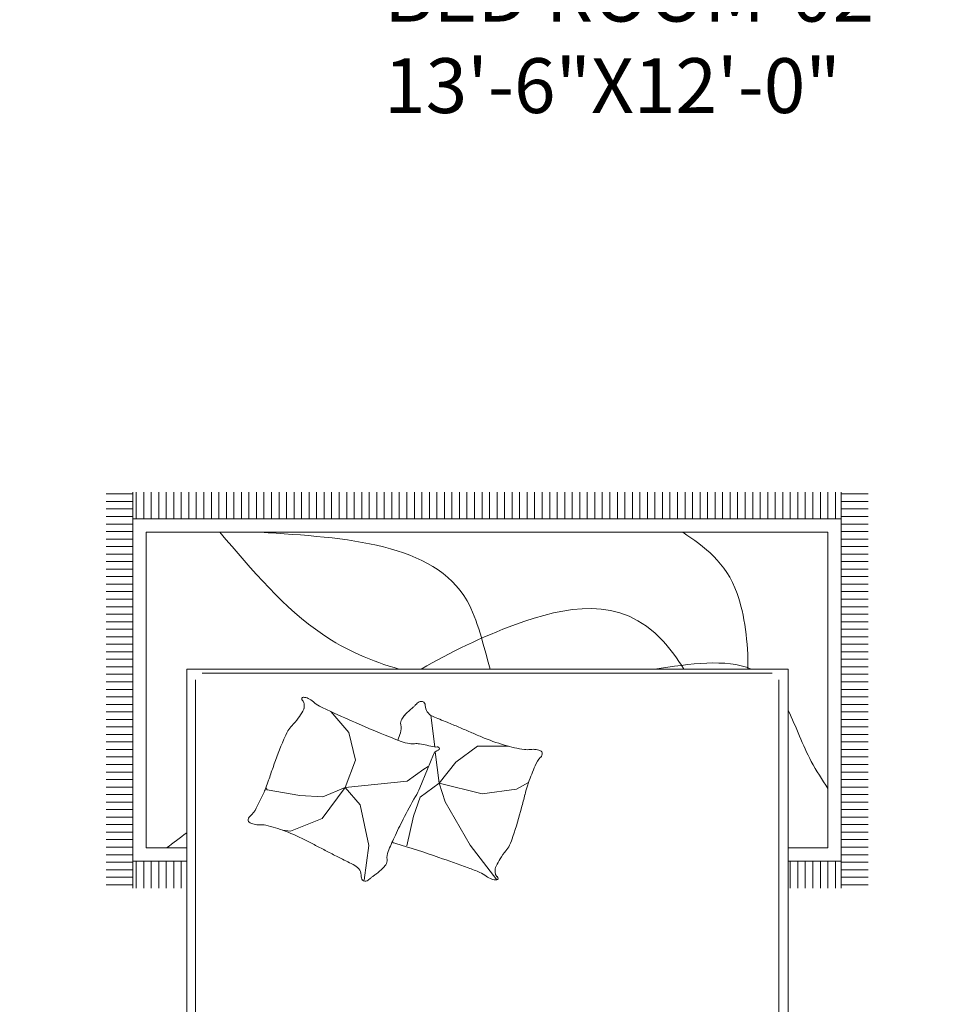
# Model space of a CAD drawing. Units: inches. Extents: x -7 to 1228, y -146 to 1091.
# Tile 18 of 88: x 425 to 511, y 103 to 194. Entities that reach past the tile are written whole.
import ezdxf

# ---------------------------------------------------------------- set-up
doc = ezdxf.new("R2010")
doc.units = ezdxf.units.IN
doc.layers.add('A-AREA-IDEN', color=7, linetype='Continuous', lineweight=18)
doc.layers.add('A-FURN', color=8, linetype='Continuous', lineweight=18)
doc.styles.add('DIM_FONT', font='SIMPLEX.shx', dxfattribs={"width": 0.8})
doc.styles.get("Standard").update_dxf_attribs({"font": 'arial.ttf'})

# ---------------------------------------------------------------- blocks, each defined once
blk = doc.blocks.new('A$C4F634EDD')
for p, q in [((0, 2.6295), (0, 2.2295)), ((0.5, 2.6295), (0, 2.6295)), ((0.5, 2.6295), (2.3, 2.6295)), ((0.5, 0.5295), (0.5, 2.6295)), ((0.5, 2.2295), (0.5, 2.6295)), ((2.3, 2.6295), (2.3, 0.5295)), ((2.3, 2.6295), (2.8, 2.6295)), ((2.3, 2.2295), (2.3, 2.6295)), ((2.8, 2.6295), (2.8, 2.2295)), ((0.2457, 2.5697), (0.2457, 2.4733)), ((0.5, 2.5771), (2.3, 2.5771)), ((2.392, 2.5115), (2.5692, 2.5765)), ((2.5692, 2.5765), (2.574, 2.5743)), ((2.574, 2.5743), (2.6638, 2.3298)), ((2.4946, 2.5331), (2.4985, 2.5445)), ((2.4985, 2.5445), (2.5516, 2.564)), ((2.5062, 2.5454), (2.5004, 2.5392)), ((2.5004, 2.5392), (2.5013, 2.5315)), ((2.5062, 2.5454), (2.5487, 2.561)), ((2.5235, 2.5256), (2.5062, 2.5454)), ((2.5483, 2.5347), (2.5487, 2.561)), ((2.5487, 2.561), (2.5571, 2.56)), ((2.5615, 2.5536), (2.5514, 2.5318)), ((2.5516, 2.564), (2.5637, 2.5584)), ((2.5571, 2.56), (2.5615, 2.5536)), ((2.5615, 2.5536), (2.5791, 2.5058)), ((2.5637, 2.5584), (2.6418, 2.3458)), ((2.3898, 2.5066), (2.392, 2.5115)), ((2.4795, 2.2621), (2.3898, 2.5066)), ((2.412, 2.5007), (2.4634, 2.5196)), ((2.4634, 2.5196), (2.4875, 2.454)), ((2.4842, 2.5232), (2.47, 2.518)), ((2.47, 2.518), (2.472, 2.5127)), ((2.472, 2.5127), (2.4862, 2.5179)), ((2.4881, 2.5126), (2.4739, 2.5074)), ((2.4739, 2.5074), (2.4759, 2.502)), ((2.4759, 2.502), (2.4901, 2.5073)), ((2.4862, 2.5179), (2.4842, 2.5232)), ((2.4901, 2.5073), (2.4881, 2.5126)), ((2.5734, 2.3187), (2.4946, 2.5331)), ((2.5013, 2.5315), (2.5188, 2.4836)), ((2.5013, 2.5315), (2.5231, 2.5214)), ((2.5231, 2.5214), (2.5235, 2.5256)), ((2.5523, 2.4417), (2.5231, 2.5214)), ((2.5483, 2.5347), (2.5235, 2.5256)), ((2.5514, 2.5318), (2.5483, 2.5347)), ((2.5807, 2.4521), (2.5514, 2.5318)), ((2.5791, 2.5058), (2.5788, 2.4956)), ((2.4361, 2.4352), (2.412, 2.5007)), ((2.492, 2.5019), (2.4778, 2.4967)), ((2.4778, 2.4967), (2.4798, 2.4914)), ((2.4798, 2.4914), (2.494, 2.4966)), ((2.4959, 2.4913), (2.4817, 2.4861)), ((2.4817, 2.4861), (2.4837, 2.4808)), ((2.4837, 2.4808), (2.4979, 2.486)), ((2.4998, 2.4807), (2.4856, 2.4755)), ((2.494, 2.4966), (2.492, 2.5019)), ((2.4979, 2.486), (2.4959, 2.4913)), ((2.5018, 2.4754), (2.4998, 2.4807)), ((2.5188, 2.4836), (2.5256, 2.4761)), ((2.5788, 2.4956), (2.5767, 2.4848)), ((2.5767, 2.4848), (2.5795, 2.4717)), ((2.4875, 2.454), (2.4361, 2.4352)), ((2.4856, 2.4755), (2.4876, 2.4702)), ((2.4876, 2.4702), (2.5018, 2.4754)), ((2.5037, 2.47), (2.4895, 2.4648)), ((2.4895, 2.4648), (2.4915, 2.4595)), ((2.4915, 2.4595), (2.5057, 2.4647)), ((2.5057, 2.4647), (2.5037, 2.47)), ((2.5256, 2.4761), (2.5342, 2.4692)), ((2.5342, 2.4692), (2.5405, 2.4574)), ((2.5405, 2.4574), (2.547, 2.4397)), ((2.5795, 2.4717), (2.586, 2.454)), ((2.5807, 2.4521), (2.6158, 2.3564)), ((2.5984, 2.4204), (2.586, 2.454)), ((0.0957, 2.4197), (0.192, 2.4197)), ((0.2994, 2.4197), (0.3957, 2.4197)), ((2.4457, 2.4146), (2.4563, 2.4185)), ((2.4563, 2.4185), (2.4602, 2.4078)), ((2.4634, 2.4211), (2.474, 2.425)), ((2.4673, 2.4104), (2.4634, 2.4211)), ((2.474, 2.425), (2.4779, 2.4143)), ((2.4811, 2.4276), (2.4917, 2.4315)), ((2.485, 2.4169), (2.4811, 2.4276)), ((2.4956, 2.4208), (2.485, 2.4169)), ((2.4917, 2.4315), (2.4956, 2.4208)), ((2.5594, 2.4061), (2.547, 2.4397)), ((2.5523, 2.4417), (2.5875, 2.346)), ((2.6047, 2.4086), (2.5984, 2.4204)), ((2.4496, 2.4039), (2.4457, 2.4146)), ((2.4602, 2.4078), (2.4496, 2.4039)), ((2.4528, 2.3951), (2.4635, 2.399)), ((2.4567, 2.3844), (2.4528, 2.3951)), ((2.4674, 2.3883), (2.4567, 2.3844)), ((2.4635, 2.399), (2.4674, 2.3883)), ((2.4779, 2.4143), (2.4673, 2.4104)), ((2.4706, 2.4016), (2.4812, 2.4055)), ((2.4745, 2.3909), (2.4706, 2.4016)), ((2.4851, 2.3949), (2.4745, 2.3909)), ((2.4812, 2.4055), (2.4851, 2.3949)), ((2.4883, 2.4081), (2.4989, 2.412)), ((2.4922, 2.3975), (2.4883, 2.4081)), ((2.5028, 2.4014), (2.4922, 2.3975)), ((2.4954, 2.3886), (2.5061, 2.3925)), ((2.4993, 2.378), (2.4954, 2.3886)), ((2.4989, 2.412), (2.5028, 2.4014)), ((2.5061, 2.3925), (2.51, 2.3819)), ((2.5622, 2.393), (2.5594, 2.4061)), ((2.5601, 2.3822), (2.5622, 2.393)), ((2.6133, 2.4017), (2.6047, 2.4086)), ((2.6201, 2.3941), (2.6133, 2.4017)), ((2.6376, 2.3463), (2.6201, 2.3941)), ((2.6499, 2.3979), (2.6397, 2.3953)), ((2.6417, 2.39), (2.6488, 2.391)), ((2.6488, 2.391), (2.6538, 2.3895)), ((2.6551, 2.397), (2.6499, 2.3979)), ((2.6538, 2.3895), (2.6596, 2.388)), ((2.6627, 2.392), (2.6551, 2.397)), ((2.6596, 2.388), (2.6626, 2.3867)), ((2.6626, 2.3867), (2.6662, 2.388)), ((2.6692, 2.394), (2.6627, 2.392)), ((2.6662, 2.388), (2.6632, 2.3828)), ((2.6736, 2.3944), (2.6692, 2.394)), ((2.6765, 2.391), (2.6736, 2.3944)), ((2.6742, 2.3795), (2.6765, 2.391)), ((0.2457, 2.366), (0.2457, 2.2697)), ((2.46, 2.3756), (2.4706, 2.3795)), ((2.4639, 2.365), (2.46, 2.3756)), ((2.4745, 2.3689), (2.4639, 2.365)), ((2.4672, 2.3561), (2.4778, 2.36)), ((2.4706, 2.3795), (2.4745, 2.3689)), ((2.4777, 2.3821), (2.4883, 2.386)), ((2.4816, 2.3715), (2.4777, 2.3821)), ((2.4778, 2.36), (2.4817, 2.3494)), ((2.4922, 2.3754), (2.4816, 2.3715)), ((2.4849, 2.3626), (2.4955, 2.3665)), ((2.4888, 2.352), (2.4849, 2.3626)), ((2.4883, 2.386), (2.4922, 2.3754)), ((2.4955, 2.3665), (2.4994, 2.3559)), ((2.51, 2.3819), (2.4993, 2.378)), ((2.5026, 2.3691), (2.5132, 2.373)), ((2.5065, 2.3585), (2.5026, 2.3691)), ((2.5171, 2.3624), (2.5065, 2.3585)), ((2.5132, 2.373), (2.5171, 2.3624)), ((2.5238, 2.3769), (2.538, 2.3821)), ((2.5277, 2.3663), (2.5238, 2.3769)), ((2.5419, 2.3715), (2.5277, 2.3663)), ((2.538, 2.3821), (2.5419, 2.3715)), ((2.5598, 2.372), (2.5601, 2.3822)), ((2.5774, 2.3242), (2.5598, 2.372)), ((2.6632, 2.3828), (2.6736, 2.3744)), ((2.6736, 2.3744), (2.6922, 2.3593)), ((2.6824, 2.3858), (2.6742, 2.3795)), ((2.6873, 2.3815), (2.6824, 2.3858)), ((2.6853, 2.369), (2.6873, 2.3815)), ((2.6946, 2.376), (2.6853, 2.369)), ((2.6922, 2.3593), (2.7051, 2.3473)), ((2.6995, 2.3713), (2.6946, 2.376)), ((2.695, 2.3603), (2.6995, 2.3713)), ((2.7031, 2.3682), (2.695, 2.3603)), ((2.7096, 2.3616), (2.7031, 2.3682)), ((2.7062, 2.351), (2.7096, 2.3616)), ((0, 2.3301), (0.5, 2.3301)), ((2.8, 2.3301), (2.3, 2.3301)), ((2.4711, 2.3455), (2.4672, 2.3561)), ((2.4817, 2.3494), (2.4711, 2.3455)), ((2.4994, 2.3559), (2.4888, 2.352)), ((2.5774, 2.3242), (2.5875, 2.346)), ((2.5875, 2.346), (2.5905, 2.3431)), ((2.5905, 2.3431), (2.5901, 2.3168)), ((2.6154, 2.3522), (2.5905, 2.3431)), ((2.613, 2.3312), (2.6077, 2.3293)), ((2.6077, 2.3293), (2.6135, 2.3141)), ((2.6192, 2.3174), (2.613, 2.3312)), ((2.6153, 2.3261), (2.6327, 2.3324)), ((2.6158, 2.3564), (2.6154, 2.3522)), ((2.6154, 2.3522), (2.6327, 2.3324)), ((2.6376, 2.3463), (2.6158, 2.3564)), ((2.6369, 2.332), (2.6161, 2.3243)), ((2.6327, 2.3324), (2.6385, 2.3386)), ((2.6418, 2.3458), (2.6369, 2.332)), ((2.6385, 2.3386), (2.6376, 2.3463)), ((2.6638, 2.3298), (2.6616, 2.3249)), ((2.7051, 2.3473), (2.7079, 2.3475)), ((2.7147, 2.3578), (2.7062, 2.351)), ((2.7079, 2.3475), (2.7079, 2.3443)), ((2.7079, 2.3443), (2.727, 2.3277)), ((2.7214, 2.3517), (2.7147, 2.3578)), ((2.7196, 2.34), (2.7214, 2.3517)), ((2.7286, 2.3466), (2.7196, 2.34)), ((2.7346, 2.3423), (2.7286, 2.3466)), ((2.732, 2.3295), (2.7346, 2.3423)), ((2.7423, 2.3345), (2.732, 2.3295)), ((2.7495, 2.325), (2.7423, 2.3345)), ((2.6172, 2.3086), (2.4844, 2.2599)), ((2.5362, 2.305), (2.5185, 2.2985)), ((2.5401, 2.2944), (2.5362, 2.305)), ((2.561, 2.3141), (2.5433, 2.3076)), ((2.5433, 2.3076), (2.5472, 2.297)), ((2.5472, 2.297), (2.5649, 2.3035)), ((2.5649, 2.3035), (2.561, 2.3141)), ((2.5855, 2.3131), (2.5734, 2.3187)), ((2.5818, 2.3178), (2.5774, 2.3242)), ((2.5901, 2.3168), (2.5818, 2.3178)), ((2.6104, 2.3222), (2.5855, 2.3131)), ((2.5901, 2.3168), (2.6097, 2.324)), ((2.6135, 2.3141), (2.6244, 2.2977)), ((2.626, 2.3069), (2.6192, 2.3174)), ((2.6616, 2.3249), (2.6234, 2.3109)), ((2.6365, 2.2916), (2.626, 2.3069)), ((2.727, 2.3277), (2.7512, 2.2983)), ((2.7406, 2.3172), (2.7495, 2.325)), ((2.7519, 2.3218), (2.7406, 2.3172)), ((2.7575, 2.3144), (2.7519, 2.3218)), ((2.7526, 2.3045), (2.7575, 2.3144)), ((2.7622, 2.308), (2.7526, 2.3045)), ((2.7574, 2.2924), (2.7673, 2.2997)), ((2.7673, 2.2997), (2.7622, 2.308)), ((0.5953, 2.1912), (0.616, 2.2738)), ((1.4546, 2.1912), (1.4752, 2.2738)), ((2.5114, 2.2959), (2.4936, 2.2894)), ((2.4936, 2.2894), (2.4976, 2.2788)), ((2.4976, 2.2788), (2.5153, 2.2853)), ((2.5153, 2.2853), (2.5114, 2.2959)), ((2.5185, 2.2985), (2.5224, 2.2879)), ((2.5224, 2.2879), (2.5401, 2.2944)), ((2.6244, 2.2977), (2.6349, 2.2825)), ((2.6349, 2.2825), (2.638, 2.273)), ((2.6407, 2.2834), (2.6365, 2.2916)), ((2.6399, 2.2712), (2.6374, 2.2659)), ((2.638, 2.273), (2.6399, 2.2712)), ((2.6438, 2.2739), (2.6407, 2.2834)), ((2.6519, 2.2716), (2.6438, 2.2739)), ((2.6535, 2.2628), (2.6519, 2.2716)), ((2.7512, 2.2983), (2.756, 2.2695)), ((2.7687, 2.2905), (2.7574, 2.2924)), ((2.7587, 2.279), (2.7699, 2.2828)), ((2.7708, 2.2725), (2.7587, 2.279)), ((2.7699, 2.2828), (2.7687, 2.2905)), ((2.7706, 2.2643), (2.7708, 2.2725)), ((2.4844, 2.2599), (2.4795, 2.2621)), ((2.6374, 2.2659), (2.6398, 2.257)), ((2.6398, 2.257), (2.6509, 2.259)), ((2.6509, 2.259), (2.6431, 2.2492)), ((2.6431, 2.2492), (2.6473, 2.2398)), ((2.6473, 2.2398), (2.6592, 2.2429)), ((2.6592, 2.2429), (2.6521, 2.2314)), ((2.6636, 2.2409), (2.6535, 2.2628)), ((2.6836, 2.2287), (2.6636, 2.2409)), ((2.7459, 2.2483), (2.7284, 2.2317)), ((2.756, 2.2695), (2.7459, 2.2483)), ((2.7509, 2.2314), (2.7459, 2.2418)), ((2.7459, 2.2418), (2.7568, 2.2352)), ((2.7529, 2.2505), (2.7645, 2.2498)), ((2.7607, 2.2424), (2.7529, 2.2505)), ((2.7568, 2.2352), (2.7607, 2.2424)), ((2.759, 2.2637), (2.7706, 2.2643)), ((2.7676, 2.2559), (2.759, 2.2637)), ((2.7645, 2.2498), (2.7676, 2.2559)), ((0, 2.2295), (0.5, 2.2295)), ((2.8, 2.2295), (2.3, 2.2295)), ((2.6521, 2.2314), (2.6598, 2.2248)), ((2.6598, 2.2248), (2.6697, 2.2309)), ((2.6697, 2.2309), (2.6684, 2.219)), ((2.6684, 2.219), (2.6761, 2.2145)), ((2.6761, 2.2145), (2.6821, 2.2237)), ((2.6821, 2.2237), (2.6843, 2.2135)), ((2.7063, 2.2256), (2.6836, 2.2287)), ((2.6843, 2.2135), (2.6927, 2.2117)), ((2.6927, 2.2117), (2.6986, 2.222)), ((2.6986, 2.222), (2.7019, 2.2098)), ((2.7284, 2.2317), (2.7063, 2.2256)), ((2.7102, 2.2104), (2.7113, 2.2218)), ((2.7113, 2.2218), (2.7192, 2.2137)), ((2.7192, 2.2137), (2.7255, 2.2152)), ((2.7255, 2.2152), (2.7242, 2.2265)), ((2.7242, 2.2265), (2.7324, 2.2165)), ((2.7324, 2.2165), (2.7386, 2.2208)), ((2.7386, 2.2208), (2.7354, 2.2306)), ((2.7354, 2.2306), (2.7462, 2.2264)), ((2.7462, 2.2264), (2.7509, 2.2314)), ((0.5878, 2.1612), (0.5953, 2.1912)), ((1.4471, 2.1612), (1.4546, 2.1912)), ((2.7019, 2.2098), (2.7102, 2.2104)), ((1.5035, 2.141), (0.5458, 2.141)), ((1.5035, 2.141), (2.2716, 1.7136)), ((0.5258, 2.121), (0.5258, 0.5617)), ((1.576, 1.9433), (1.5624, 1.8479)), ((0.5458, 1.8684), (1.5653, 1.8684)), ((1.5624, 1.8479), (1.5641, 1.7178)), ((2.2716, 0.5617), (2.2716, 1.7136)), ((0.3386, 0), (0.3386, 1.1852)), ((0.3486, 1.1052), (0.3486, 1.1852)), ((0.3711, 1.1052), (0.3711, 1.1852)), ((0.3936, 1.1052), (0.3936, 1.1852)), ((0.4161, 1.1052), (0.4161, 1.1852)), ((0.4386, 1.1052), (0.4386, 1.1852)), ((0.4611, 1.1052), (0.4611, 1.1852)), ((0.4836, 1.1052), (0.4836, 1.1852)), ((2.3061, 1.1052), (2.3061, 1.1852)), ((2.3286, 1.1052), (2.3286, 1.1852)), ((2.3511, 1.1052), (2.3511, 1.1852)), ((2.3736, 1.1052), (2.3736, 1.1852)), ((2.3961, 1.1052), (2.3961, 1.1852)), ((2.4186, 1.1052), (2.4186, 1.1852)), ((2.4411, 1.1052), (2.4411, 1.1852)), ((2.4588, 1.1852), (2.4588, 0)), ((0.2586, 1.1753), (0.3386, 1.1753)), ((0.2586, 1.1528), (0.3386, 1.1528)), ((1.031, 1.1612), (1.0448, 1.0581)), ((1.4276, 1.1611), (1.3484, 1.0571)), ((2.4588, 1.1753), (2.5388, 1.1753)), ((2.4588, 1.1528), (2.5388, 1.1528)), ((0.2586, 1.1303), (0.3386, 1.1303)), ((2.4588, 1.1303), (2.5388, 1.1303)), ((0.2586, 1.1078), (0.3386, 1.1078)), ((0.3386, 1.1052), (0.5, 1.1052)), ((2.3, 1.1052), (2.4588, 1.1052)), ((2.4588, 1.1078), (2.5388, 1.1078)), ((0.2586, 1.0853), (0.3386, 1.0853)), ((0.2586, 1.0628), (0.3386, 1.0628)), ((0.3786, 1.0652), (0.5, 1.0652)), ((0.3786, 0.12), (0.3786, 1.0652)), ((2.3, 1.0652), (2.4188, 1.0652)), ((2.4188, 1.0652), (2.4188, 0.12)), ((2.4588, 1.0853), (2.5388, 1.0853)), ((2.4588, 1.0628), (2.5388, 1.0628)), ((0.2586, 1.0403), (0.3386, 1.0403)), ((1.0448, 1.0581), (1.019, 0.936)), ((1.1784, 0.9702), (1.1586, 1.0591)), ((1.3484, 1.0571), (1.2733, 0.9268)), ((2.4588, 1.0403), (2.5388, 1.0403)), ((0.2586, 1.0178), (0.3386, 1.0178)), ((0.8108, 1.0151), (0.7868, 1.0117)), ((0.9054, 0.9773), (0.8108, 1.0151)), ((2.4588, 1.0178), (2.5388, 1.0178)), ((0.2586, 0.9953), (0.3386, 0.9953)), ((0.9743, 0.8845), (0.9054, 0.9773)), ((2.4588, 0.9953), (2.5388, 0.9953)), ((0.2586, 0.9728), (0.3386, 0.9728)), ((0.2586, 0.9503), (0.3386, 0.9503)), ((1.1982, 0.9129), (1.1784, 0.9702)), ((2.4588, 0.9728), (2.5388, 0.9728)), ((2.4588, 0.9503), (2.5388, 0.9503)), ((0.2586, 0.9278), (0.3386, 0.9278)), ((1.019, 0.936), (0.9743, 0.8845)), ((1.2733, 0.9268), (1.2555, 0.8715)), ((2.4588, 0.9278), (2.5388, 0.9278)), ((0.2586, 0.9053), (0.3386, 0.9053)), ((0.7403, 0.8913), (0.737, 0.8849)), ((0.8384, 0.9085), (0.7403, 0.8913)), ((0.9072, 0.912), (0.8384, 0.9085)), ((0.9743, 0.8845), (0.9072, 0.912)), ((0.9743, 0.8845), (1.0052, 0.802)), ((0.9743, 0.8845), (1.16, 0.8656)), ((1.1973, 0.8853), (1.2203, 0.829)), ((1.2555, 0.8715), (1.1982, 0.9129)), ((1.2555, 0.8715), (1.384, 0.9031)), ((1.384, 0.9031), (1.4868, 0.8892)), ((1.4868, 0.8892), (1.5228, 0.8692)), ((2.4588, 0.9053), (2.5388, 0.9053)), ((0.2586, 0.8828), (0.3386, 0.8828)), ((0.2586, 0.8603), (0.3386, 0.8603)), ((1.16, 0.8656), (1.2099, 0.8295)), ((1.2555, 0.8715), (1.2437, 0.7773)), ((1.2555, 0.8715), (1.3049, 0.8082)), ((2.4588, 0.8828), (2.5388, 0.8828)), ((2.4588, 0.8603), (2.5388, 0.8603)), ((0.2586, 0.8378), (0.3386, 0.8378)), ((1.2099, 0.8295), (1.222, 0.8209)), ((1.2203, 0.829), (1.2381, 0.7855)), ((2.4588, 0.8378), (2.5388, 0.8378)), ((0.2586, 0.8153), (0.3386, 0.8153)), ((1.0052, 0.802), (0.9846, 0.7194)), ((1.3049, 0.8082), (1.3701, 0.7608)), ((2.4588, 0.8153), (2.5388, 0.8153)), ((0.2586, 0.7928), (0.3386, 0.7928)), ((0.2586, 0.7703), (0.3386, 0.7703)), ((2.4588, 0.7928), (2.5388, 0.7928)), ((2.4588, 0.7703), (2.5388, 0.7703)), ((0.2586, 0.7478), (0.3386, 0.7478)), ((1.2419, 0.7626), (1.23, 0.668)), ((1.3701, 0.7608), (1.463, 0.7608)), ((2.4588, 0.7478), (2.5388, 0.7478)), ((0.2586, 0.7253), (0.3386, 0.7253)), ((0.9846, 0.7194), (0.931, 0.6569)), ((2.4588, 0.7253), (2.5388, 0.7253)), ((0.2586, 0.7028), (0.3386, 0.7028)), ((0.2586, 0.6803), (0.3386, 0.6803)), ((2.4588, 0.7028), (2.5388, 0.7028)), ((2.4588, 0.6803), (2.5388, 0.6803)), ((0.2586, 0.6578), (0.3386, 0.6578)), ((2.4588, 0.6578), (2.5388, 0.6578)), ((0.2586, 0.6353), (0.3386, 0.6353)), ((2.4588, 0.6353), (2.5388, 0.6353)), ((0.2586, 0.6128), (0.3386, 0.6128)), ((0.2586, 0.5903), (0.3386, 0.5903)), ((2.4588, 0.6128), (2.5388, 0.6128)), ((2.4588, 0.5903), (2.5388, 0.5903)), ((0.2586, 0.5678), (0.3386, 0.5678)), ((2.4588, 0.5678), (2.5388, 0.5678)), ((0.2586, 0.5453), (0.3386, 0.5453)), ((0.5458, 0.5417), (2.2516, 0.5417)), ((2.4588, 0.5453), (2.5388, 0.5453)), ((0.2586, 0.5228), (0.3386, 0.5228)), ((2.3, 0.5295), (0.5, 0.5295)), ((2.4588, 0.5228), (2.5388, 0.5228)), ((0.2586, 0.5003), (0.3386, 0.5003)), ((0.2586, 0.4778), (0.3386, 0.4778)), ((2.4588, 0.5003), (2.5388, 0.5003)), ((2.4588, 0.4778), (2.5388, 0.4778)), ((0.2586, 0.4553), (0.3386, 0.4553)), ((2.4588, 0.4553), (2.5388, 0.4553)), ((0.2586, 0.4328), (0.3386, 0.4328)), ((2.4588, 0.4328), (2.5388, 0.4328)), ((0.2586, 0.4103), (0.3386, 0.4103)), ((0.2586, 0.3878), (0.3386, 0.3878)), ((2.4588, 0.4103), (2.5388, 0.4103)), ((2.4588, 0.3878), (2.5388, 0.3878)), ((0.2586, 0.3653), (0.3386, 0.3653)), ((2.4588, 0.3653), (2.5388, 0.3653)), ((0.2586, 0.3428), (0.3386, 0.3428)), ((2.4588, 0.3428), (2.5388, 0.3428)), ((0.2586, 0.3203), (0.3386, 0.3203)), ((0.2586, 0.2978), (0.3386, 0.2978)), ((2.4588, 0.3203), (2.5388, 0.3203)), ((2.4588, 0.2978), (2.5388, 0.2978)), ((0.2586, 0.2753), (0.3386, 0.2753)), ((2.4588, 0.2753), (2.5388, 0.2753)), ((0.2586, 0.2528), (0.3386, 0.2528)), ((2.4588, 0.2528), (2.5388, 0.2528)), ((0.2586, 0.2303), (0.3386, 0.2303)), ((0.2586, 0.2078), (0.3386, 0.2078)), ((2.4588, 0.2303), (2.5388, 0.2303)), ((2.4588, 0.2078), (2.5388, 0.2078)), ((0.2586, 0.1853), (0.3386, 0.1853)), ((2.4588, 0.1853), (2.5388, 0.1853)), ((0.2586, 0.1628), (0.3386, 0.1628)), ((2.4588, 0.1628), (2.5388, 0.1628)), ((0.2586, 0.1403), (0.3386, 0.1403)), ((2.4188, 0.12), (0.3786, 0.12)), ((2.4588, 0.1403), (2.5388, 0.1403)), ((0.2586, 0.1178), (0.3386, 0.1178)), ((0.2586, 0.0953), (0.3386, 0.0953)), ((2.4588, 0.1178), (2.5388, 0.1178)), ((2.4588, 0.0953), (2.5388, 0.0953)), ((0.2586, 0.0728), (0.3386, 0.0728)), ((2.4588, 0.08), (0.3386, 0.08)), ((0.3486, 0), (0.3486, 0.08)), ((0.3711, 0), (0.3711, 0.08)), ((0.3936, 0), (0.3936, 0.08)), ((0.4161, 0), (0.4161, 0.08)), ((0.4386, 0), (0.4386, 0.08)), ((0.4611, 0), (0.4611, 0.08)), ((0.4836, 0), (0.4836, 0.08)), ((0.5061, 0), (0.5061, 0.08)), ((0.5286, 0), (0.5286, 0.08)), ((0.5511, 0), (0.5511, 0.08)), ((0.5736, 0), (0.5736, 0.08)), ((0.5961, 0), (0.5961, 0.08)), ((0.6186, 0), (0.6186, 0.08)), ((0.6411, 0), (0.6411, 0.08)), ((0.6636, 0), (0.6636, 0.08)), ((0.6861, 0), (0.6861, 0.08)), ((0.7086, 0), (0.7086, 0.08)), ((0.7311, 0), (0.7311, 0.08)), ((0.7536, 0), (0.7536, 0.08)), ((0.7761, 0), (0.7761, 0.08)), ((0.7986, 0), (0.7986, 0.08)), ((0.8211, 0), (0.8211, 0.08)), ((0.8436, 0), (0.8436, 0.08)), ((0.8661, 0), (0.8661, 0.08)), ((0.8886, 0), (0.8886, 0.08)), ((0.9111, 0), (0.9111, 0.08)), ((0.9336, 0), (0.9336, 0.08)), ((0.9561, 0), (0.9561, 0.08)), ((0.9786, 0), (0.9786, 0.08)), ((1.0011, 0), (1.0011, 0.08)), ((1.0236, 0), (1.0236, 0.08)), ((1.0461, 0), (1.0461, 0.08)), ((1.0686, 0), (1.0686, 0.08)), ((1.0911, 0), (1.0911, 0.08)), ((1.1136, 0), (1.1136, 0.08)), ((1.1361, 0), (1.1361, 0.08)), ((1.1586, 0), (1.1586, 0.08)), ((1.1811, 0), (1.1811, 0.08)), ((1.2036, 0), (1.2036, 0.08)), ((1.2261, 0), (1.2261, 0.08)), ((1.2486, 0), (1.2486, 0.08)), ((1.2711, 0), (1.2711, 0.08)), ((1.2936, 0), (1.2936, 0.08)), ((1.3161, 0), (1.3161, 0.08)), ((1.3386, 0), (1.3386, 0.08)), ((1.3611, 0), (1.3611, 0.08)), ((1.3836, 0), (1.3836, 0.08)), ((1.4061, 0), (1.4061, 0.08)), ((1.4286, 0), (1.4286, 0.08)), ((1.4511, 0), (1.4511, 0.08)), ((1.4736, 0), (1.4736, 0.08)), ((1.4961, 0), (1.4961, 0.08)), ((1.5186, 0), (1.5186, 0.08)), ((1.5411, 0), (1.5411, 0.08)), ((1.5636, 0), (1.5636, 0.08)), ((1.5861, 0), (1.5861, 0.08)), ((1.6086, 0), (1.6086, 0.08)), ((1.6311, 0), (1.6311, 0.08)), ((1.6536, 0), (1.6536, 0.08)), ((1.6761, 0), (1.6761, 0.08)), ((1.6986, 0), (1.6986, 0.08)), ((1.7211, 0), (1.7211, 0.08)), ((1.7436, 0), (1.7436, 0.08)), ((1.7661, 0), (1.7661, 0.08)), ((1.7886, 0), (1.7886, 0.08)), ((1.8111, 0), (1.8111, 0.08)), ((1.8336, 0), (1.8336, 0.08)), ((1.8561, 0), (1.8561, 0.08)), ((1.8786, 0), (1.8786, 0.08)), ((1.9011, 0), (1.9011, 0.08)), ((1.9236, 0), (1.9236, 0.08)), ((1.9461, 0), (1.9461, 0.08)), ((1.9686, 0), (1.9686, 0.08)), ((1.9911, 0), (1.9911, 0.08)), ((2.0136, 0), (2.0136, 0.08)), ((2.0361, 0), (2.0361, 0.08)), ((2.0586, 0), (2.0586, 0.08)), ((2.0811, 0), (2.0811, 0.08)), ((2.1036, 0), (2.1036, 0.08)), ((2.1261, 0), (2.1261, 0.08)), ((2.1486, 0), (2.1486, 0.08)), ((2.1711, 0), (2.1711, 0.08)), ((2.1936, 0), (2.1936, 0.08)), ((2.2161, 0), (2.2161, 0.08)), ((2.2386, 0), (2.2386, 0.08)), ((2.2611, 0), (2.2611, 0.08)), ((2.2836, 0), (2.2836, 0.08)), ((2.3061, 0), (2.3061, 0.08)), ((2.3286, 0), (2.3286, 0.08)), ((2.3511, 0), (2.3511, 0.08)), ((2.3736, 0), (2.3736, 0.08)), ((2.3961, 0), (2.3961, 0.08)), ((2.4186, 0), (2.4186, 0.08)), ((2.4411, 0), (2.4411, 0.08)), ((2.4588, 0.0728), (2.5388, 0.0728)), ((0.2586, 0.0503), (0.3386, 0.0503)), ((2.4588, 0.0503), (2.5388, 0.0503)), ((0.2586, 0.0278), (0.3386, 0.0278)), ((0.2586, 0.0053), (0.3386, 0.0053)), ((2.4588, 0.0278), (2.5388, 0.0278)), ((2.4588, 0.0053), (2.5388, 0.0053))]:
    blk.add_line(p, q)
for radius in [0.1222, 0.0865]:
    blk.add_circle((0.2457, 2.4197), radius)
for centre, radius, start, end in [((0.5848, 2.5274), 0.0131, 101.2724, 206.5805), ((0.5999, 2.4516), 0.0904, 90, 101.2724), ((0.5999, 2.3808), 0.1611, 81.5628, 90), ((0.5788, 2.2388), 0.3048, 74.256, 81.5628), ((1.3132, 2.5864), 0.0539, 275.2592, 300.6513), ((1.3554, 2.5152), 0.0289, 85.6975, 120.6513), ((1.3556, 2.519), 0.0251, 68.2117, 85.6975), ((1.3634, 2.533), 0.00428, 78.1069, 158.0096), ((1.3647, 2.5395), 0.00232, 258.1069, 19.564), ((1.3637, 2.5391), 0.00342, 19.564, 68.2117), ((1.444, 2.5274), 0.0131, 101.2724, 206.5805), ((1.4591, 2.4516), 0.0904, 90, 101.2724), ((1.4591, 2.3808), 0.1611, 81.5628, 90), ((1.438, 2.2388), 0.3048, 74.256, 81.5628), ((2.1724, 2.5864), 0.0539, 275.2592, 300.6513), ((2.2146, 2.5152), 0.0289, 85.6975, 120.6513), ((2.2149, 2.519), 0.0251, 68.2117, 85.6975), ((2.2226, 2.533), 0.00428, 78.1069, 158.0096), ((2.224, 2.5395), 0.00232, 258.1069, 19.564), ((2.2229, 2.5391), 0.00342, 19.564, 68.2117), ((0.6036, 2.5368), 0.0342, 206.5805, 265.5998), ((0.7272, 2.7653), 0.2422, 254.256, 262.4531), ((0.7851, 3.2019), 0.6827, 262.4531, 270), ((0.7851, 3.5682), 1.049, 270, 276.0867), ((0.8402, 3.0514), 0.5293, 276.0867, 280.1899), ((1.1602, -8.1346), 10.6675, 90.30153, 91.21582), ((1.1169, 2.2433), 0.2897, 85.1982, 92.5386), ((1.2142, 3.4021), 0.8732, 265.1982, 269.4243), ((1.4317, 2.2032), 0.3916, 128.3886, 133.8115), ((1.2362, 2.45), 0.0768, 117.2396, 128.3886), ((1.3082, 2.3102), 0.234, 110.8603, 117.2396), ((1.2204, 4.0232), 1.4943, 269.4243, 271.9079), ((1.2995, 2.4357), 0.0992, 126.0864, 143.8234), ((1.2995, 2.4357), 0.0992, 105.9352, 126.0864), ((1.2429, 3.3501), 0.8208, 271.9079, 275.2592), ((1.2995, 2.4357), 0.0992, 85.7841, 105.9352), ((1.3739, 2.5288), 0.0156, 158.0096, 201.421), ((1.1177, 2.5413), 0.246, 347.8905, 351.8665), ((1.3288, 2.5111), 0.0328, 351.8665, 21.421), ((1.4628, 2.5368), 0.0342, 206.5805, 265.5998), ((1.5865, 2.7653), 0.2422, 254.256, 262.4531), ((1.6443, 3.2019), 0.6827, 262.4531, 270), ((1.6443, 3.5682), 1.049, 270, 276.0867), ((1.4785, 15.4878), 12.9656, 271.22425, 272.05324), ((1.97, 2.3805), 0.1524, 92.5386, 100.1899), ((1.9761, 2.2433), 0.2897, 85.1982, 92.5386), ((2.0734, 3.4021), 0.8732, 265.1982, 269.4243), ((2.291, 2.2032), 0.3916, 128.3886, 133.8115), ((2.0954, 2.45), 0.0768, 117.2396, 128.3886), ((2.1674, 2.3102), 0.234, 110.8603, 117.2396), ((2.0797, 4.0232), 1.4943, 269.4243, 271.9079), ((2.1588, 2.4357), 0.0992, 126.0864, 143.8234), ((2.1588, 2.4357), 0.0992, 105.9352, 126.0864), ((2.1021, 3.3501), 0.8208, 271.9079, 275.2592), ((2.1588, 2.4357), 0.0992, 85.7841, 105.9352), ((2.2331, 2.5288), 0.0156, 158.0096, 201.421), ((1.977, 2.5413), 0.246, 347.8905, 351.8665), ((2.1881, 2.5111), 0.0328, 351.8665, 21.421), ((1.0898, 2.4496), 0.4918, 173.7676, 180), ((0.5462, 2.4142), 0.0899, 41.4429, 53.7359), ((0.5368, 2.3783), 0.1399, 45.0976, 62.7964), ((0.5368, 2.3783), 0.1399, 27.3988, 45.0976), ((1.3165, 2.3233), 0.2252, 133.8115, 140.9651), ((1.2995, 2.4357), 0.0992, 143.8234, 161.5603), ((1.5522, 2.448), 0.1983, 167.8905, 172.3191), ((1.949, 2.4496), 0.4918, 173.7676, 180), ((2.1757, 2.3233), 0.2252, 133.8115, 140.9651), ((2.1588, 2.4357), 0.0992, 143.8234, 161.5603), ((2.4114, 2.448), 0.1983, 167.8905, 172.3191), ((0.8019, 2.4496), 0.204, 180, 189.6844), ((0.5741, 2.4389), 0.0526, 25.3551, 41.4429), ((0.4851, 2.3967), 0.1511, 21.8149, 25.3551), ((0.4345, 2.3765), 0.2056, 18.7799, 21.8149), ((1.3127, 2.3625), 0.2002, 151.6832, 156.9972), ((1.1799, 2.4341), 0.0493, 140.9651, 151.6832), ((2.2605, 2.3525), 0.9131, 172.3191, 176.6313), ((1.6611, 2.4496), 0.204, 180, 189.6844), ((2.1719, 2.3625), 0.2002, 151.6832, 156.9972), ((2.0391, 2.4341), 0.0493, 140.9651, 151.6832), ((3.1198, 2.3525), 0.9131, 172.3191, 176.6313), ((0.576, 2.4246), 0.0562, 0, 18.7799), ((0.5406, 2.4246), 0.0915, 345.3149, 0), ((0.5368, 2.3783), 0.1399, 16.515, 27.3988), ((0.5368, 2.3783), 0.1399, 5.6311, 16.515), ((1.4703, 2.5637), 0.882, 189.6844, 192.1984), ((2.0266, 2.3663), 0.6787, 176.6313, 181.6331), ((2.3295, 2.5637), 0.882, 189.6844, 192.1984), ((2.8858, 2.3663), 0.6787, 176.6313, 181.6331), ((0.2982, 2.3103), 0.3171, 8.0051, 12.1984), ((1.1575, 2.3103), 0.3171, 8.0051, 12.1984), ((-0.0401, 2.2627), 0.6588, 2.6649, 8.0051), ((2.7128, 2.3859), 1.3652, 181.6331, 183.055), ((0.8191, 2.2627), 0.6588, 2.6649, 8.0051), ((3.5721, 2.3859), 1.3652, 181.6331, 183.055), ((14.9657, 3.0398), 13.6356, 183.05496, 183.50486), ((15.8249, 3.0398), 13.6356, 183.05496, 183.50486), ((0.5503, 2.2902), 0.0677, 345.9548, 2.6649), ((1.4096, 2.2902), 0.0677, 345.9548, 2.6649), ((1.1303, 1.9835), 0.2721, 85.9172, 93.5552), ((1.1455, 2.197), 0.058, 69.3257, 85.9172), ((0.9871, 1.7772), 0.5066, 65.6735, 69.3257), ((0.473, 2.8815), 0.7387, 293.4844, 295.3111), ((0.6058, 0.9338), 1.4323, 63.5015, 65.6735), ((1.1054, 1.9358), 0.3126, 57.865, 63.5015), ((1.3322, 2.8815), 0.7387, 293.4844, 295.3111), ((0.473, 2.8815), 0.7387, 287.1982, 289.428), ((0.473, 2.8815), 0.7387, 289.428, 291.6577), ((0.473, 2.8815), 0.7387, 291.6577, 293.4844), ((0.8841, 1.5835), 0.7286, 54.1737, 57.865), ((1.6762, 2.2258), 0.3212, 183.5049, 189.9984), ((1.3322, 2.8815), 0.7387, 287.1982, 289.428), ((1.3322, 2.8815), 0.7387, 289.428, 291.6577), ((1.3322, 2.8815), 0.7387, 291.6577, 293.4844), ((2.5355, 2.2258), 0.3212, 183.5049, 189.9984), ((0.5887, 2.1609), 0.000917, 165.9551, 274.0829), ((0.5695, 2.4301), 0.2708, 274.0829, 279.4841), ((0.5763, 2.3896), 0.2297, 279.4841, 287.3864), ((0.6807, 2.0561), 0.1197, 96.4341, 107.3864), ((0.6836, 2.0301), 0.1459, 78.4414, 96.4341), ((0.759, 2.3985), 0.2301, 258.4414, 272.7491), ((0.7026, 3.5718), 1.4048, 272.7491, 274.6176), ((0.9136, 0.9591), 1.2165, 92.6096, 94.6176), ((1.2501, -19.8405), 22.0183, 90.37908, 91.01965), ((1.2012, -3.5404), 5.7185, 89.7135, 90.9704), ((1.224, 1.0141), 1.164, 86.426, 89.7135), ((1.2875, 2.0302), 0.1459, 77.131, 86.426), ((1.3099, 2.1283), 0.0453, 62.7159, 77.131), ((1.3658, 2.2367), 0.0767, 242.7159, 253.7788), ((1.3688, 2.247), 0.0875, 253.7788, 262.8796), ((1.3581, 2.1615), 0.00132, 262.8796, 343.3022), ((1.3409, 2.1667), 0.0193, 343.3022, 9.9984), ((1.448, 2.1609), 0.000917, 165.9551, 274.0829), ((1.4288, 2.4301), 0.2708, 274.0829, 279.4841), ((1.4355, 2.3896), 0.2297, 279.4841, 287.3864), ((1.5399, 2.0561), 0.1197, 96.4341, 107.3864), ((1.5429, 2.0301), 0.1459, 78.4414, 96.4341), ((1.6182, 2.3985), 0.2301, 258.4414, 272.7491), ((1.5619, 3.5718), 1.4048, 272.7491, 274.6176), ((1.7729, 0.9591), 1.2165, 92.6096, 94.6176), ((2.1093, -19.8405), 22.0183, 90.37908, 91.01965), ((2.0605, -3.5404), 5.7185, 89.7135, 90.9704), ((2.0833, 1.0141), 1.164, 86.426, 89.7135), ((2.1467, 2.0302), 0.1459, 77.131, 86.426), ((2.1691, 2.1283), 0.0453, 62.7159, 77.131), ((2.2251, 2.2367), 0.0767, 242.7159, 253.7788), ((2.2281, 2.247), 0.0875, 253.7788, 262.8796), ((2.2174, 2.1615), 0.00132, 262.8796, 343.3022), ((2.2001, 2.1667), 0.0193, 343.3022, 9.9984), ((0.5458, 2.121), 0.02, 90, 180), ((1.2147, 1.9017), 0.3751, 20.1488, 39.6445), ((1.3977, 1.9688), 0.1801, 351.8644, 20.1488), ((0.5458, 1.8884), 0.02, 180, 270), ((2.0378, 1.5789), 0.1942, 97.7304, 103.1904), ((2.0195, 1.7137), 0.0581, 79.2724, 97.7304), ((1.2737, -2.2227), 4.0646, 77.0745, 79.2724), ((0.6102, 18.0525), 16.3521, 273.75703, 274.62393), ((1.4194, 4.2174), 2.5158, 281.6741, 283.1904), ((1.0582, 5.4638), 3.7801, 277.692, 279.495), ((2.0359, 1.0981), 0.6574, 74.0648, 77.0745), ((1.7125, -0.0344), 1.8351, 72.2636, 74.0648), ((0.9863, 1.1494), 0.0359, 297.2902, 3.2455), ((1.0348, 1.1521), 0.0127, 51.1864, 183.2455), ((0.9991, 1.1077), 0.0697, 45.8726, 51.1864), ((1.0791, 1.1902), 0.0452, 225.8726, 232.4713), ((1.2846, 1.4577), 0.3825, 232.4713, 233.7837), ((1.4338, 1.1026), 0.0601, 110.3452, 128.5854), ((1.4251, 1.1259), 0.0352, 86.0516, 110.3452), ((1.4376, 1.1398), 0.0142, 126.5792, 169.5926), ((1.4273, 1.1567), 0.00443, 13.2808, 86.0516), ((1.4254, 1.1562), 0.0063, 306.5792, 13.2808), ((0.6683, 0.6162), 0.6605, 52.7849, 53.7837), ((0.9362, 0.9689), 0.2176, 46.4776, 52.7849), ((1.0327, 1.0706), 0.0774, 35.8936, 46.4776), ((-0.4107, 5.9078), 5.0942, 289.0836, 290.1287), ((1.0543, 1.9106), 0.8371, 290.1287, 292.7069), ((1.3469, 1.2115), 0.0792, 292.7069, 308.5854), ((1.4996, 1.1284), 0.0771, 169.5926, 177.2714), ((1.4378, 1.1314), 0.0153, 177.2714, 194.5709), ((1.4611, 1.1374), 0.0393, 194.5709, 206.8179), ((1.8575, -0.7096), 2.0162, 116.4147, 117.4999), ((-0.4173, 3.8699), 3.0972, 296.4147, 297.2902), ((1.0771, 1.1027), 0.0226, 351.9508, 35.8936), ((1.1449, 1.0931), 0.0458, 171.9508, 202.4162), ((0.2266, 4.0657), 3.145, 286.6085, 289.0836), ((1.7401, 1.2785), 0.352, 206.8179, 210.9056), ((1.6045, 1.1973), 0.194, 210.9056, 219.7005), ((-1.8336, 6.2238), 5.8383, 297.49208, 297.84822), ((3.744, -4.3336), 6.1019, 117.49986, 117.84822), ((2.032, 1.4591), 1.0054, 202.4162, 205.0529), ((1.3929, 1.0217), 0.081, 26.0735, 39.7005), ((0.5736, 1.5979), 0.6236, 290.7486, 297.4921), ((1.0922, 1.1636), 0.1166, 280.7366, 286.6085), ((2.6493, 1.7476), 1.6868, 205.0529, 207.0884), ((1.2892, 0.9709), 0.1965, 17.8396, 26.0735), ((0.6422, 1.4168), 0.43, 282.6252, 290.7486), ((-0.4304, 0.4175), 2.003, 15.2625, 17.8396), ((0.6894, 0.9832), 0.0058, 121.6917, 179.0386), ((0.7004, 0.983), 0.0168, 179.0386, 229.4914), ((0.7131, 0.9448), 0.0509, 103.0402, 121.6917), ((0.7152, 0.9361), 0.0599, 86.6119, 103.0402), ((0.7224, 1.0587), 0.063, 266.6119, 282.6252), ((2.541, 1.6922), 1.5652, 207.0884, 209.936), ((0.6405, 0.9128), 0.0755, 26.3332, 49.4914), ((-1.6775, -0.2344), 2.6619, 25.1732, 26.3332), ((-0.0881, 0.5109), 1.6481, 13.841, 15.2625), ((0.5689, 0.8213), 0.1798, 20.7081, 25.1732), ((0.2268, 0.692), 0.5454, 18.2369, 20.7081), ((0.9989, 0.8042), 0.2143, 22.2355, 29.936), ((2.0418, 1.0357), 0.5454, 193.841, 196.3122), ((2.3102, 1.3785), 1.6481, 198.2369, 199.6584), ((1.6908, 0.933), 0.1798, 196.3122, 200.7773), ((4.0115, 1.8135), 2.6619, 200.7773, 201.9373), ((2.6444, 1.4979), 2.003, 199.6584, 202.2355), ((1.6124, 0.8472), 0.0755, 201.9373, 225.0955), ((1.2594, 0.7942), 0.0231, 202.2355, 252.8133), ((1.2512, 0.7678), 0.00467, 289.3799, 72.8133), ((1.5721, 0.3449), 0.43, 98.2293, 106.3527), ((1.5195, 0.708), 0.063, 82.216, 98.2293), ((1.5362, 0.8298), 0.0599, 262.216, 278.6443), ((1.5375, 0.8209), 0.0509, 278.6443, 297.2959), ((1.5473, 0.7819), 0.0168, 354.6428, 45.0955), ((1.5582, 0.7808), 0.0058, 297.2959, 354.6428), ((0.9722, 0.8143), 0.1965, 202.2355, 210.4694), ((2.2689, -2.1899), 3.145, 111.0043, 113.4795), ((0.1831, 0.4093), 1.0054, 18.0203, 19.3448), ((1.1834, 0.6373), 0.1166, 98.1216, 111.0043), ((1.1763, 0.687), 0.0663, 85.4882, 98.1216), ((1.1871, 0.8241), 0.0712, 265.4882, 277.6784), ((1.1727, 0.9313), 0.1794, 277.6784, 284.8807), ((1.2689, 0.569), 0.1955, 97.9822, 104.8807), ((1.2465, 0.729), 0.034, 85.7407, 97.9822), ((1.2497, 0.772), 0.0092, 265.7407, 289.3799), ((1.6266, 0.159), 0.6236, 106.3527, 113.0962), ((0.8727, 0.7557), 0.081, 210.4694, 224.0964), ((1.0957, 0.7061), 0.0458, 347.5549, 18.0203), ((-1.0798, 6.3161), 6.1019, 293.10398, 293.45234), ((3.6722, -4.6377), 5.8383, 113.0962, 113.45234), ((0.6752, 0.5644), 0.194, 35.3015, 44.0964), ((3.0455, -3.9778), 5.0942, 113.4795, 114.5246), ((1.1625, 0.6914), 0.0226, 167.5549, 211.4977), ((1.2092, 0.72), 0.0774, 211.4977, 222.0817), ((2.4404, -2.1823), 3.0972, 112.0188, 112.8944), ((0.5234, 2.5582), 2.0162, 292.0188, 293.104), ((0.5462, 0.4731), 0.352, 31.2138, 35.3015), ((0.8136, 0.6351), 0.0393, 18.9668, 31.2138), ((1.2784, -0.1047), 0.8371, 114.5246, 117.1028), ((1.3133, 0.814), 0.2176, 222.0817, 228.389), ((1.6074, 1.1451), 0.6605, 228.389, 229.3878), ((1.2495, 0.6379), 0.0359, 112.8944, 178.8496), ((0.8506, 0.6191), 0.0063, 130.9751, 197.6767), ((0.8372, 0.6345), 0.0142, 310.9751, 353.9885), ((0.8364, 0.6429), 0.0153, 1.6673, 18.9668), ((0.7746, 0.6411), 0.0771, 353.9885, 1.6673), ((0.8382, 0.6719), 0.0601, 294.7411, 312.9813), ((0.9332, 0.57), 0.0792, 117.1028, 132.9813), ((0.9284, 0.3533), 0.3825, 48.0754, 49.3878), ((1.1538, 0.6043), 0.0452, 41.4767, 48.0754), ((1.2399, 0.6804), 0.0697, 221.4767, 226.7905), ((1.2009, 0.6389), 0.0127, 226.7905, 358.8496), ((0.8488, 0.6185), 0.00443, 197.6767, 270.4475), ((0.8486, 0.6493), 0.0352, 270.4475, 294.7411)]:
    blk.add_arc(centre, radius, start, end)
for points in [[(0.4393, 1.0652), (0.4595, 1.05), (0.4798, 1.0348), (0.5, 1.0195)], [(1.9003, 0.5295), (2.0065, 0.514), (2.1132, 0.4978), (2.1894, 0.5295)]]:
    blk.add_open_spline(points, degree=3)
for points, knots in [([(2.3, 0.6535), (2.3236, 0.7026), (2.3554, 0.7914), (2.4015, 0.8608), (2.4188, 0.8868)], [1893.525221, 1893.525221, 1893.525221, 1893.525221, 2051.902476, 2146.74457, 2146.74457, 2146.74457, 2146.74457]), ([(0.5992, 0.12), (0.6957, 0.2341), (0.8523, 0.4189), (1.0536, 0.5069), (1.136, 0.5295)], [0, 0, 0, 0, 432.822832, 701.445452, 701.445452, 701.445452, 701.445452]), ([(0.7187, 0.12), (0.9791, 0.1362), (1.326, 0.1577), (1.3868, 0.4574), (1.408, 0.5295)], [0, 0, 0, 0, 653.160442, 870.050857, 870.050857, 870.050857, 870.050857]), ([(1.2016, 0.5295), (1.2892, 0.479), (1.5144, 0.3684), (1.8265, 0.2994), (1.9681, 0.4992), (1.9875, 0.5295)], [936.534237, 936.534237, 936.534237, 936.534237, 1243.285375, 1683.261222, 1758.254386, 1758.254386, 1758.254386, 1758.254386]), ([(2.1796, 0.5295), (2.1798, 0.4519), (2.1548, 0.2369), (2.0487, 0.164), (1.9846, 0.12)], [2202.034493, 2202.034493, 2202.034493, 2202.034493, 2357.807635, 2594.446174, 2594.446174, 2594.446174, 2594.446174])]:
    blk.add_open_spline(points, degree=3, knots=knots)
at = {"style": 'DIM_FONT', "width": 0.8, "flags": 9}
for tag, p in [('YSIZE', (0.5, 2.6295)), ('XSIZE', (0.5, 2.6295)), ('XSIZE', (2.2985, 2.6295)), ('YSIZE', (2.2985, 2.6295))]:
    blk.add_attdef(tag, p, '', height=0.0005, dxfattribs=at)

msp = doc.modelspace()

# ---------------------------------------------------------------- block references
at = {"layer": 'A-FURN', "xscale": -30.79356024027943, "yscale": 30.79356024027943, "zscale": 30.79356024027943, "rotation": 180}
msp.add_blockref('A$C4F634EDD', (424.889, 149.972), dxfattribs=at)

# ---------------------------------------------------------------- texts
at = {"layer": 'A-AREA-IDEN', "insert": (458.471, 198.413), "char_height": 5.05676, "attachment_point": 1}
msp.add_mtext_dynamic_manual_height_columns('BED ROOM-02\\P13\'-6"X12\'-0"', width=137.28212, gutter_width=25.284, heights=[0], dxfattribs=at)

doc.saveas('drawing.dxf')
